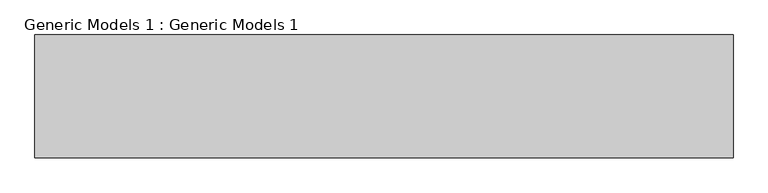
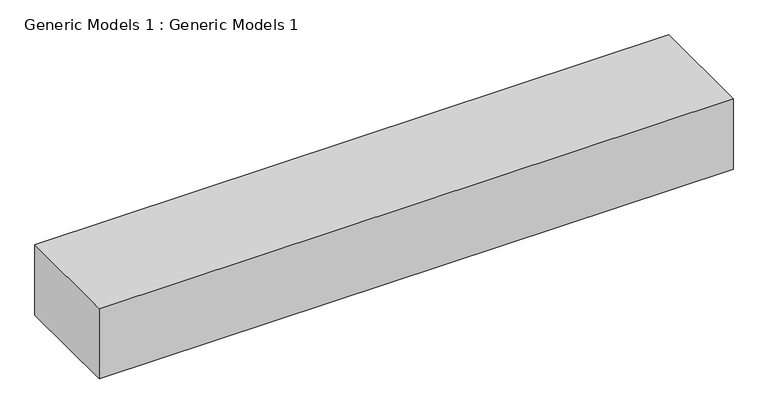
"""IFC4 building model written with IfcOpenShell, lengths in millimetres: proxy geometry, Generic Models 1 : Generic Models 1."""

from ifc_helpers import new_model, si_unit, frame, origin, place, context, project, spatial, polyline, outline, extrude, source, transform, mapped, element, save


def generic_models_1_generic_models_1_82b812d9(model_context):
    return source(origin(), model_context, "Body", "SweptSolid", [
        extrude(outline(polyline([(4979.9930105, -7244.2747571), (4979.9930105, -9047.5192661), (-5281.6069895, -9047.5192661), (-5281.6069895, -7244.2747571), (4979.9930105, -7244.2747571)])), frame((0.0, 0.0, 6400.8), z_axis=(0.0, 0.0, 1.0), x_axis=(1.0, 0.0, 0.0)), (0.0, 0.0, 1.0), 1201.7484148),
    ])


if __name__ == "__main__":
    model = new_model("IFC4")
    model_context = context("Model", 3, world=origin())
    ifc_project = project(units=[si_unit("LENGTHUNIT", "METRE", prefix="MILLI")], contexts=[model_context])
    site = spatial("IfcSite", under=ifc_project)
    building = spatial("IfcBuilding", under=site)
    placement = place(None, origin())
    generic_models_1_generic_models_1_shape = generic_models_1_generic_models_1_82b812d9(model_context)
    element("IfcBuildingElementProxy", 1, Name="Generic Models 1 : Generic Models 1", ObjectType="Generic Models 1 : Generic Models 1", at=placement, inside=building, context=model_context, shape_type="MappedRepresentation", body=[
        mapped(generic_models_1_generic_models_1_shape, transform((0.0, 0.0, 0.0), x_axis=(1.0, 0.0, 0.0), y_axis=(0.0, 1.0, 0.0), z_axis=(0.0, 0.0, 1.0))),
    ])
    save(model, "model.ifc")
